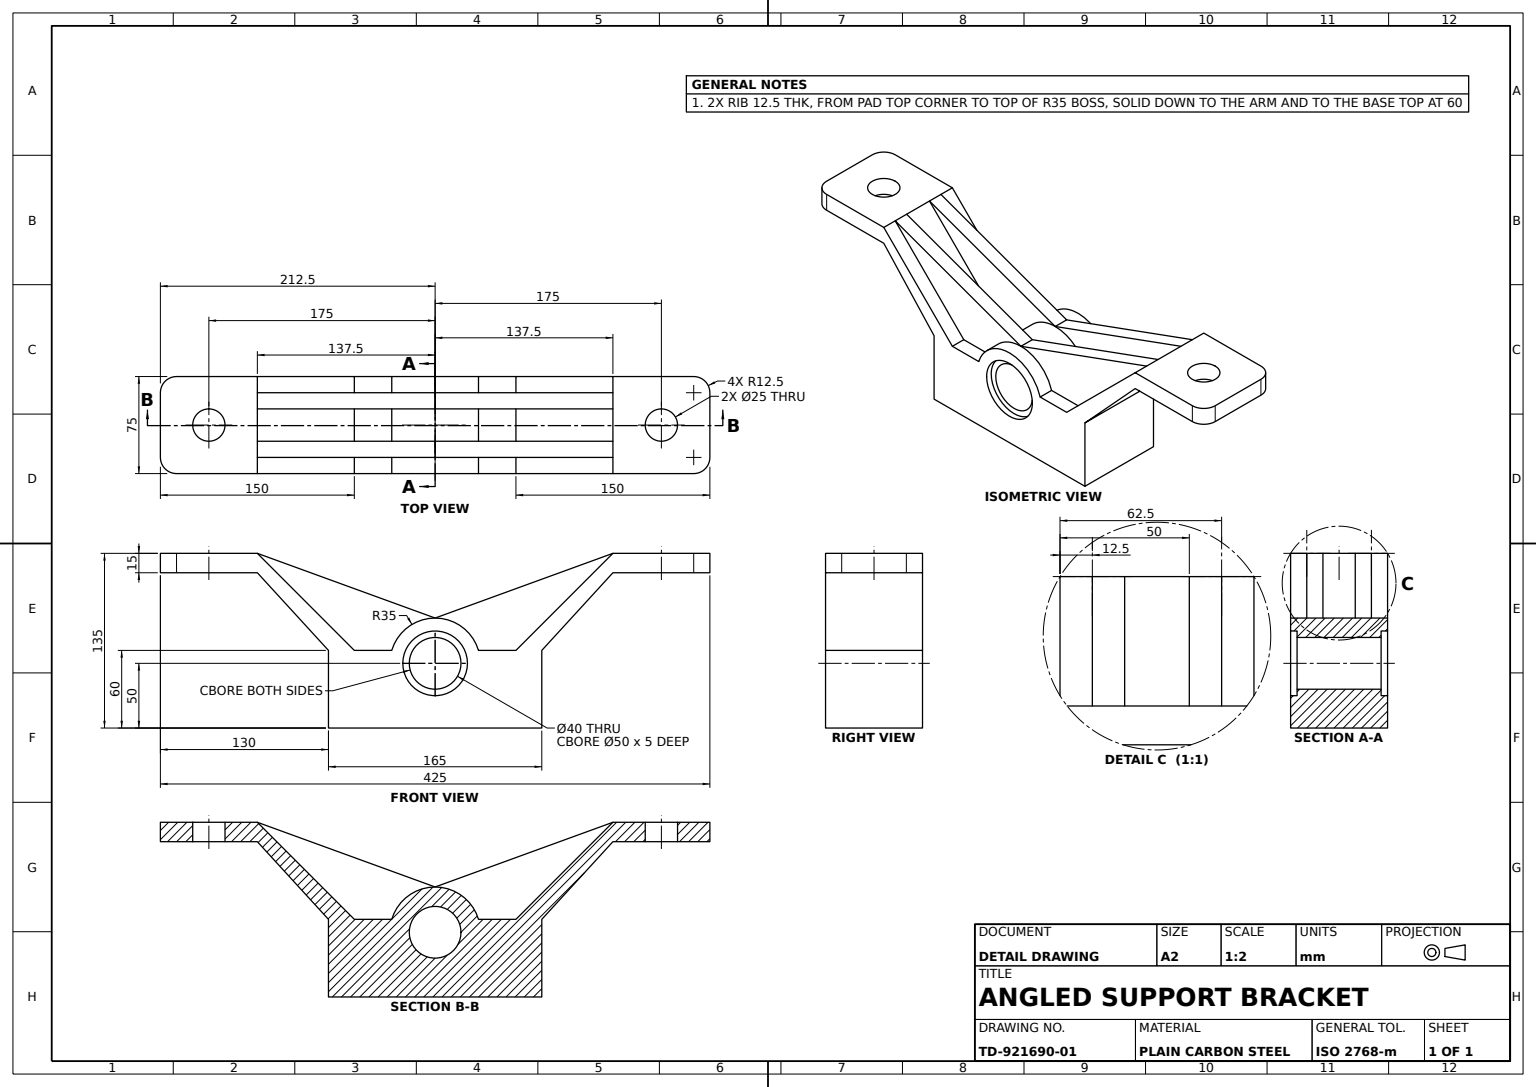
from build123d import *

# Parameters (mm, degrees)
SUPPORT_BODY_DEPTH           = 75
RIB_FRONT_DEPTH              = 12.5
RIB_START                    = -12.5
RIB_BACK_DEPTH               = 12.5
MOUNTING_HOLES_SKETCH_R      = 12.5
MOUNTING_HOLES_2X_25_DEPTH   = 108.5
FLANGE_FILLET_R12_5_A_R      = 12.5
FLANGE_FILLET_R12_5_B_R      = 12.5
FLANGE_FILLET_R12_5_C_R      = 12.5
FLANGE_FILLET_R12_5_D_R      = 12.5
COUNTERBORE_FRONT_SKETCH_R   = 25
COUNTERBORE_FRONT_50X5_DEPTH = 5
SHAFT_BORE_SKETCH_R          = 20
SHAFT_BORE_40_DEPTH          = 98
COUNTERBORE_START            = -5
COUNTERBORE_BACK_SKETCH_R    = 25
COUNTERBORE_BACK_50X5_DEPTH  = 5


with BuildPart() as part:
    # Support Profile Sketch → Support Body (new body)
    with BuildSketch(Plane.XY):
        with BuildLine():
            Line((33.541019662, 30), (62.5, 30))
            Line((62.5, 30), (137.5, 105))
            Line((137.5, 105), (212.5, 105))
            Line((212.5, 105), (212.5, 90))
            Line((212.5, 90), (137.5, 90))
            Line((137.5, 90), (82.5, 30))
            Line((82.5, 30), (82.5, 0))
            Line((82.5, 0), (82.5, -30))
            Line((82.5, -30), (-82.5, -30))
            Line((-82.5, -30), (-82.5, 30))
            Line((-82.5, 30), (-137.5, 90))
            Line((-137.5, 90), (-212.5, 90))
            Line((-212.5, 90), (-212.5, 105))
            Line((-212.5, 105), (-137.5, 105))
            Line((-137.5, 105), (-62.5, 30))
            Line((-62.5, 30), (-33.541019662, 30))
            ThreePointArc((-33.541019662, 30), (0, 55), (33.541019662, 30))
        make_face()
    extrude(amount=-SUPPORT_BODY_DEPTH)

    # Rib Front Sketch → Rib Front (add)
    with BuildSketch(Plane.XY.offset(-12.5)):
        with BuildLine():
            Line((137.5, 105), (0, 55))
            ThreePointArc((0, 55), (20.916500663, 48.062430401), (33.541019662, 30))
            Line((33.541019662, 30), (62.5, 30))
            Line((62.5, 30), (137.5, 105))
        make_face()
        with BuildLine():
            ThreePointArc((-33.541019662, 30), (-20.916500663, 48.062430401), (0, 55))
            Line((0, 55), (-137.5, 105))
            Line((-137.5, 105), (-62.5, 30))
            Line((-62.5, 30), (-33.541019662, 30))
        make_face()
    extrude(amount=-RIB_FRONT_DEPTH)

    # Rib Back Sketch → Rib Back (add)
    with BuildSketch(Plane(origin=(0, 0, -62.5), x_dir=(-1, 0, 0), z_dir=(0, 0, -1)).offset(RIB_START)):
        with BuildLine():
            Line((137.5, 105), (0, 55))
            ThreePointArc((0, 55), (20.916500663, 48.062430401), (33.541019662, 30))
            Line((33.541019662, 30), (62.5, 30))
            Line((62.5, 30), (137.5, 105))
        make_face()
        with BuildLine():
            Line((0, 55), (-137.5, 105))
            Line((-137.5, 105), (-62.5, 30))
            Line((-62.5, 30), (-33.541019662, 30))
            ThreePointArc((-33.541019662, 30), (-20.916500663, 48.062430401), (0, 55))
        make_face()
    extrude(amount=RIB_BACK_DEPTH)

    # Mounting Holes Sketch → Mounting Holes 2xØ25 (cut)
    with BuildSketch(Plane(origin=(0, 105, 0), x_dir=(1, 0, 0), z_dir=(0, 1, 0))):
        with Locations(Location((175, 37.5, 0), (0, 0, 270))):
            Circle(MOUNTING_HOLES_SKETCH_R)
        with Locations(Location((-175, 37.5, 0), (0, 0, 90))):
            Circle(MOUNTING_HOLES_SKETCH_R)
    extrude(amount=-MOUNTING_HOLES_2X_25_DEPTH, mode=Mode.SUBTRACT)

    # Flange Fillet R12.5 A
    flange_fillet_r12_5_a_edges = [part.edges().sort_by_distance(p)[0] for p in [
        (212.5, 97.5, 0),
    ]]
    fillet(flange_fillet_r12_5_a_edges, radius=FLANGE_FILLET_R12_5_A_R)

    # Flange Fillet R12.5 B
    flange_fillet_r12_5_b_edges = [part.edges().sort_by_distance(p)[0] for p in [
        (212.5, 97.5, -75),
    ]]
    fillet(flange_fillet_r12_5_b_edges, radius=FLANGE_FILLET_R12_5_B_R)

    # Flange Fillet R12.5 C
    flange_fillet_r12_5_c_edges = [part.edges().sort_by_distance(p)[0] for p in [
        (-212.5, 97.5, -75),
    ]]
    fillet(flange_fillet_r12_5_c_edges, radius=FLANGE_FILLET_R12_5_C_R)

    # Flange Fillet R12.5 D
    flange_fillet_r12_5_d_edges = [part.edges().sort_by_distance(p)[0] for p in [
        (-212.5, 97.5, 0),
    ]]
    fillet(flange_fillet_r12_5_d_edges, radius=FLANGE_FILLET_R12_5_D_R)

    # Counterbore Front Sketch → Counterbore Front Ø50x5 (cut)
    with BuildSketch(Plane.XY):
        with Locations((0, 20)):
            Circle(COUNTERBORE_FRONT_SKETCH_R)
    extrude(amount=-COUNTERBORE_FRONT_50X5_DEPTH, mode=Mode.SUBTRACT)

    # Shaft Bore Sketch → Shaft Bore Ø40 (cut)
    with BuildSketch(Plane.XY.offset(-5)):
        with Locations((0, 20)):
            Circle(SHAFT_BORE_SKETCH_R)
    extrude(amount=-SHAFT_BORE_40_DEPTH, mode=Mode.SUBTRACT)

    # Counterbore Back Sketch → Counterbore Back Ø50x5 (cut)
    with BuildSketch(Plane(origin=(0, 0, -75), x_dir=(-1, 0, 0), z_dir=(0, 0, -1)).offset(COUNTERBORE_START)):
        with Locations(Location((0, 20, 0), (0, 0, 180))):
            Circle(COUNTERBORE_BACK_SKETCH_R)
    extrude(amount=COUNTERBORE_BACK_50X5_DEPTH, mode=Mode.SUBTRACT)


solid = part.part
